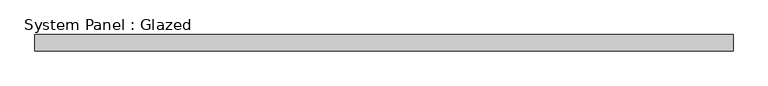
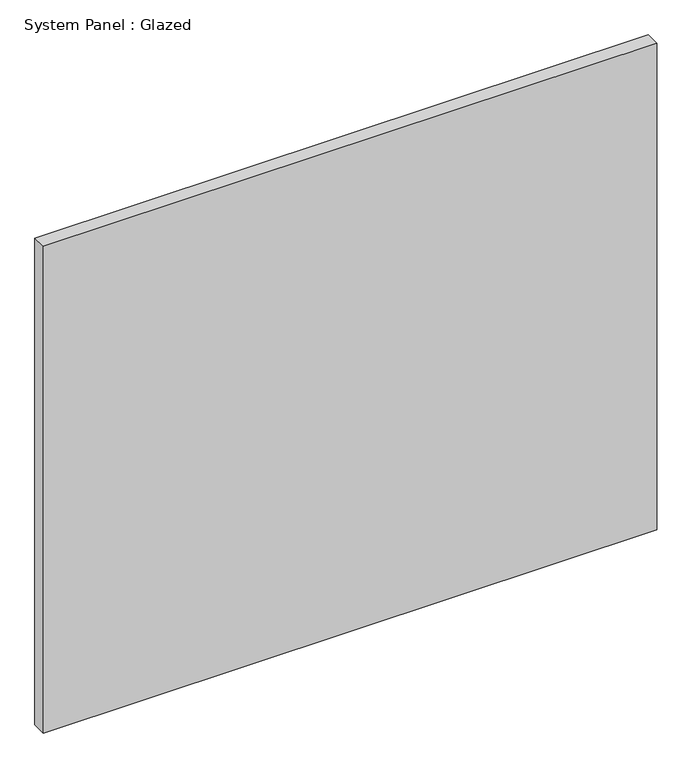
"""IFC4 building model written with IfcOpenShell, lengths in millimetres: plate geometry, System Panel : Glazed."""

from ifc_helpers import new_model, si_unit, origin, origin_with_axes, place, context, project, spatial, polyline, outline, extrude, source, transform, mapped, element, save


def system_panel_glazed_7a42c5f5(model_context):
    return source(origin(), model_context, "Body", "SweptSolid", [
        extrude(outline(polyline([(540.67075, 19.05), (-540.67075, 19.05), (-540.67075, 44.45), (540.67075, 44.45), (540.67075, 19.05)])), origin_with_axes(), (0.0, 0.0, 1.0), 907.161),
    ])


if __name__ == "__main__":
    model = new_model("IFC4")
    model_context = context("Model", 3, world=origin())
    ifc_project = project(units=[si_unit("LENGTHUNIT", "METRE", prefix="MILLI")], contexts=[model_context])
    site = spatial("IfcSite", under=ifc_project)
    building = spatial("IfcBuilding", under=site)
    placement = place(None, origin())
    system_panel_glazed_shape = system_panel_glazed_7a42c5f5(model_context)
    element("IfcPlate", 1, ObjectType="System Panel : Glazed", at=placement, inside=building, context=model_context, shape_type="MappedRepresentation", body=[
        mapped(system_panel_glazed_shape, transform((0.0, 0.0, 0.0), x_axis=(1.0, 0.0, 0.0), y_axis=(0.0, 1.0, 0.0), z_axis=(0.0, 0.0, 1.0))),
    ])
    save(model, "model.ifc")

# Revit data of these elements
# Type "System Panel : Glazed"
#   Construction Type Id = "GSP4R"
#   Analytic Construction = "1/8 in Pilkington single glazing"
#   Visual Light Transmittance = 0.9
#   Solar Heat Gain Coefficient = 0.86
#   Heat Transfer Coefficient (U) = 1.18115 BTU/(h·ft²·°F)
#   Define Thermal Properties by = 1
# Element 1 (IfcPlate, "System Panel : Glazed")
#   Materials on its faces: "Glass"
# Materials
#   "Glass": class "Glass", colour RGB 0 128 192, transparency 0.75, Description = "Soda Lime Glass", Cost = 0
